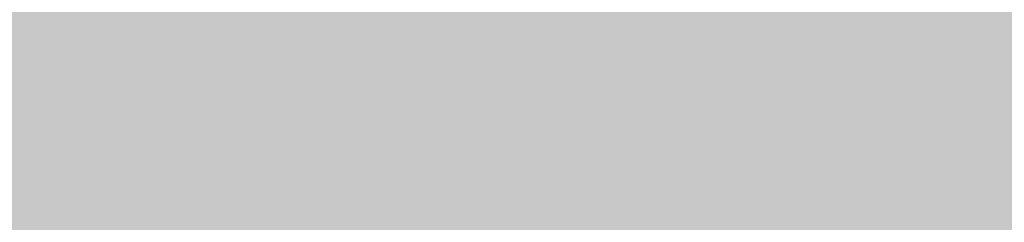
# Model space of a CAD drawing. Units: feet. Extents: x 3168 to 4724, y 827 to 1477.
# Tile 216 of 256: x 3363.87 to 3379.08, y 1093.65 to 1096.78. Entities that reach past the tile are written whole.
import ezdxf

# ---------------------------------------------------------------- set-up
doc = ezdxf.new("R2010")
doc.units = ezdxf.units.FT
doc.layers.add('A-ELEV-PATT', color=8, linetype='Continuous', lineweight=13)

msp = doc.modelspace()

# ---------------------------------------------------------------- hatches: boundary and pattern name
at = {"layer": 'A-ELEV-PATT'}
h = msp.add_hatch(color=256, dxfattribs=at)
h.dxf.hatch_style = 1
edge = h.paths.add_edge_path()
edge.add_ellipse((3552.906, 979.22), major_axis=(36.745, 0), ratio=0.484848, start_angle=0, end_angle=360)
edge = h.paths.add_edge_path()
edge.add_ellipse((3559.892, 929.252), major_axis=(36.745, 0), ratio=0.484848, start_angle=0, end_angle=360)
edge = h.paths.add_edge_path()
edge.add_line((3299.317, 1198.606), (3479.917, 1198.606))
edge.add_line((3479.917, 1198.606), (3479.917, 1209.869))
edge.add_spline(control_points=[(3479.917, 1209.869), (3464.301, 1209.869), (3448.686, 1209.869), (3410.949, 1209.869), (3388.828, 1209.869), (3355.647, 1209.869), (3344.586, 1209.869), (3327.996, 1209.869), (3322.466, 1209.869), (3314.17, 1209.869), (3311.405, 1209.869), (3307.257, 1209.869), (3305.875, 1209.869), (3303.801, 1209.869), (3303.11, 1209.869), (3302.073, 1209.869), (3301.727, 1209.869), (3301.209, 1209.869), (3301.036, 1209.869), (3300.777, 1209.869), (3300.69, 1209.869), (3300.561, 1209.869), (3300.517, 1209.869), (3300.453, 1209.869), (3300.431, 1209.869), (3300.399, 1209.869), (3300.388, 1209.869), (3300.366, 1209.869), (3300.346, 1209.869), (3300.346, 1209.869), (3300.346, 1209.869), (3300.343, 1209.869), (3300.341, 1209.869), (3300.338, 1209.869), (3300.337, 1209.869), (3300.334, 1209.869), (3300.332, 1209.869), (3300.326, 1209.869), (3300.321, 1209.869), (3300.311, 1209.869), (3300.306, 1209.869), (3300.291, 1209.869), (3300.28, 1209.869), (3300.232, 1209.869), (3300.195, 1209.869), (3299.951, 1209.871), (3299.745, 1209.874), (3299.437, 1209.883), (3299.334, 1209.887), (3299.181, 1209.893), (3299.13, 1209.895), (3298.652, 1209.917), (3298.229, 1209.946), (3297.602, 1210.002), (3297.393, 1210.023), (3297.083, 1210.058), (3296.979, 1210.07), (3296.293, 1210.155), (3295.718, 1210.243), (3294.869, 1210.399), (3294.588, 1210.454), (3294.169, 1210.543), (3294.03, 1210.574), (3291.707, 1211.101), (3289.654, 1211.813), (3285.776, 1213.564), (3283.951, 1214.603), (3280.512, 1216.98), (3278.897, 1218.318), (3276.38, 1220.829), (3275.416, 1221.918), (3274.039, 1223.708), (3273.581, 1224.35), (3273.143, 1225.016)], knot_values=[39.119033, 39.119033, 39.119033, 39.119033, 39.286353, 39.286353, 39.523379, 39.523379, 39.641892, 39.641892, 39.701148, 39.701148, 39.730777, 39.730777, 39.745591, 39.745591, 39.752998, 39.752998, 39.756701, 39.756701, 39.758553, 39.758553, 39.759479, 39.759479, 39.759942, 39.759942, 39.760173, 39.760173, 39.760289, 39.760289, 39.760405, 39.760405, 39.760463, 39.760463, 39.763389, 39.763389, 39.764851, 39.764851, 39.767304, 39.767304, 39.773825, 39.773825, 39.78057, 39.78057, 39.79477, 39.79477, 39.845194, 39.845194, 40.126715, 40.126715, 40.267476, 40.267476, 40.337856, 40.337856, 40.927023, 40.927023, 41.221606, 41.221606, 41.368898, 41.368898, 42.202622, 42.202622, 42.619485, 42.619485, 42.827916, 42.827916, 46.118323, 46.118323, 49.408731, 49.408731, 52.699139, 52.699139, 54.927489, 54.927489, 56.104228, 56.104228, 56.104228, 56.104228], weights=[1, 1, 1, 1, 1, 1, 1, 1, 1, 1, 1, 1, 1, 1, 1, 1, 1, 1, 1, 1, 1, 1, 1, 1, 1, 1, 1, 1, 1, 1, 1, 1, 1, 1, 1, 1, 1, 1, 1, 1, 1, 1, 1, 1, 1, 1, 1, 1, 1, 1, 1, 1, 1, 1, 1, 1, 1, 1, 1, 1, 1, 1, 1, 1, 1, 1, 1, 1, 1, 1, 1, 1, 1, 1], degree=3, periodic=0)
edge.add_line((3273.143, 1225.016), (3273.143, 1099.016))
edge.add_line((3273.143, 1099.016), (3299.317, 1099.016))
edge.add_line((3299.317, 1099.016), (3299.317, 1198.606))
edge = h.paths.add_edge_path()
edge.add_line((3304.758, 1324.158), (3479.917, 1324.158))
edge.add_line((3479.917, 1324.158), (3479.917, 1335.715))
edge.add_line((3479.917, 1335.715), (3269.162, 1335.715))
edge.add_spline(control_points=[(3269.162, 1335.715), (3264.024, 1335.715), (3258.364, 1328.958), (3259.264, 1323.9)], knot_values=[0, 0, 0, 0, 15.412191, 15.412191, 15.412191, 15.412191], degree=3, periodic=0)
edge.add_line((3259.264, 1323.9), (3265.517, 1288.769))
edge.add_line((3265.517, 1288.769), (3275.265, 1261.546))
edge.add_line((3275.265, 1261.546), (3304.758, 1261.546))
edge.add_line((3304.758, 1261.546), (3304.758, 1324.158))
h = msp.add_hatch(color=256, dxfattribs=at)
h.dxf.hatch_style = 1
h.paths.add_polyline_path([(3384.525, 1099.016), (3335.029, 1099.016), (3299.317, 1099.016), (3273.143, 1099.016), (3217.565, 1099.016), (3168.069, 827.116), (3335.029, 827.116)])

doc.saveas('drawing.dxf')
